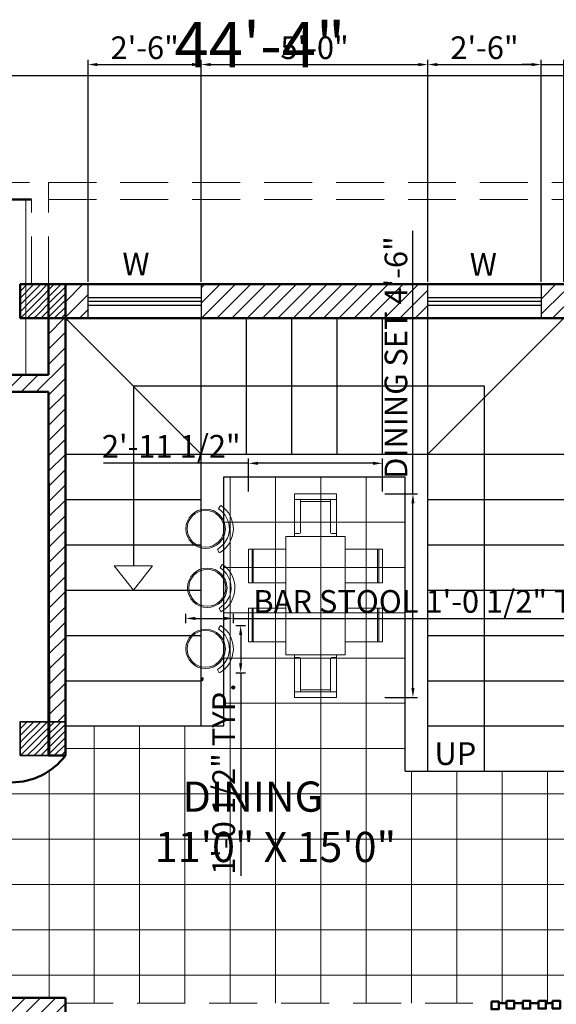
# Model space of a CAD drawing. Units: millimetres. Extents: x 225995 to 227247, y 225507 to 226008.
# Tile 3 of 23: x 226236 to 226378, y 225743 to 226004. Entities that reach past the tile are written whole.
import ezdxf

# ---------------------------------------------------------------- set-up
doc = ezdxf.new("R2010")
doc.units = ezdxf.units.MM
doc.linetypes.add('DASHED', pattern=[19.05, 12.7, -6.35])
for name, color, linetype, lineweight in [('A-ANNO-DIMS', 2, 'Continuous', 18), ('A-ANNO-TEXT', 3, 'Continuous', 18), ('A-AREA-IDEN', 30, 'Continuous', 18), ('A-COLS', 40, 'Continuous', 35), ('A-FLOR-PATT', 8, 'Continuous', 13), ('A-FLOR-STRS', 141, 'Continuous', 25), ('A-FURN', 9, 'Continuous', 18), ('A-GLAZ', 4, 'Continuous', 25), ('A-WALL', 7, 'Continuous', 50), ('A-WALL-OVHD', 1, 'DASHED', 18), ('A-WALL-PATT', 8, 'Continuous', 13)]:
    doc.layers.add(name, color=color, linetype=linetype, lineweight=lineweight)
doc.styles.get("Standard").update_dxf_attribs({"font": 'arial.ttf'})
doc.dimstyles.new('ISO-25', dxfattribs={"dimtxt": 6, "dimasz": 2.5, "dimexe": 1.25, "dimexo": 0.625, "dimtad": 1, "dimdec": 0, "dimlunit": 3, "dimtxsty": 'Standard', "dimcen": 2.5, "dimadec": 0, "dimazin": 0, "dimtfac": 1, "dimtdec": 0, "dimtmove": 0, "dimatfit": 3, "dimfxl": 1, "dimarcsym": 0})
pattern_1 = [(45, (-144, 118.1361), (-0.898025612, 0.898025612), [])]
pattern_2 = [(45, (-144, 234), (-0.898025612, 0.898025612), [])]

# ---------------------------------------------------------------- blocks, each defined once
blk = doc.blocks.new('A$C2A521B94')
for p, q in [((-548, 0, -343), (-548, 441, -343)), ((-548, 441, -343), (-150, 441, -343)), ((-548, 398, -343), (-150, 398, -343)), ((-548, 385, -343), (-150, 385, -343)), ((-150, 441, -343), (-150, 0, -343)), ((548, 441, -343), (150, 441, -343)), ((150, 441, -343), (150, 0, -343)), ((548, 398, -343), (150, 398, -343)), ((548, 385, -343), (150, 385, -343)), ((548, 0, -343), (548, 441, -343)), ((700, 0), (-700, 0)), ((-700, 0), (-700, -700)), ((700, -700), (700, 0)), ((-700, -103), (-1204, -103)), ((-1204, -103), (-1204, -597)), ((-1137, -103), (-1137, -597)), ((-733, -103), (-733, -157)), ((700, -103), (1204, -103)), ((733, -103), (733, -157)), ((1137, -103), (1137, -597)), ((1204, -103), (1204, -597)), ((-748, -172), (-1137, -172)), ((-1113, -172), (-1113, -528)), ((748, -172), (1137, -172)), ((1113, -172), (1113, -528)), ((-748, -528), (-1137, -528)), ((-733, -597), (-733, -543)), ((733, -597), (733, -543)), ((748, -528), (1137, -528)), ((-1204, -597), (-700, -597)), ((1204, -597), (700, -597)), ((-700, -700), (700, -700)), ((-548, -700, -343), (-548, -1141, -343)), ((-150, -1141, -343), (-150, -700, -343)), ((150, -1141, -343), (150, -700, -343)), ((548, -700, -343), (548, -1141, -343)), ((-548, -1085, -343), (-150, -1085, -343)), ((-548, -1098, -343), (-150, -1098, -343)), ((-548, -1141, -343), (-150, -1141, -343)), ((548, -1085, -343), (150, -1085, -343)), ((548, -1098, -343), (150, -1098, -343)), ((548, -1141, -343), (150, -1141, -343))]:
    blk.add_line(p, q)
for centre, start, end in [((-748, -157), 270, 0), ((748, -157), 180, 270), ((-748, -543), 0, 90), ((748, -543), 90, 180)]:
    blk.add_arc(centre, 14.7, start, end)
blk = doc.blocks.new('A$C2872593E')
for p, q in [((35, 351), (0, 373)), ((471, 339), (508, 360))]:
    blk.add_line(p, q)
for radius in [212, 198]:
    blk.add_circle((250, 213), radius)
for centre, radius, start, end in [((250, 213), 298, 29.6321, 146.9853), ((250, 213), 255, 29.6321, 147.1495), ((1, 374), 0.85, 146.9853, 237.1495), ((1, 374), 0.85, 146.9853, 237.1495)]:
    blk.add_arc(centre, radius, start, end)
at = {"flags": 9}
for tag in ['ZSIZE', 'YSIZE', 'XSIZE']:
    blk.add_attdef(tag, (257, 228), '', height=0.5, rotation=178.4267, dxfattribs=at)
blk = doc.blocks.new('A$C005B7AE8')
for p, q in [((0, 0.7), (0, 0.57)), ((0.03, 0.71), (0.03, 0.58)), ((0.46, 0.74), (0.04, 0.74)), ((0.44, 0.74), (0.06, 0.74)), ((0.38, 0.48), (0.12, 0.48)), ((0.13, 0.5), (0.15, 0.5)), ((0.14, 0.49), (0.14, 0.52)), ((0.14, 0.48), (0.14, 0.5)), ((0.15, 0.5), (0.15, 0.48)), ((0.35, 0.5), (0.35, 0.48)), ((0.37, 0.5), (0.35, 0.5)), ((0.36, 0.49), (0.36, 0.52)), ((0.36, 0.48), (0.36, 0.5)), ((0.47, 0.71), (0.47, 0.58)), ((0.5, 0.7), (0.5, 0.57))]:
    blk.add_line(p, q)
for centre in [(0.14, 0.55), (0.36, 0.55)]:
    blk.add_circle(centre, 0.00582)
for centre, radius, start, end in [((0.04, 0.7), 0.04, 90, 180), ((0.92, 0.57), 0.916, 179.9528, 200.6123), ((0.15, 0.45), 0.158, 140.1815, 162.8478), ((0.06, 0.71), 0.03, 90, 180), ((0.04, 0.58), 0.01, 180, 265.0115), ((0.25, 2.99), 2.42, 265.0115, 274.9885), ((0.14, 0.5), 0.00615, 5.1568, 174.8432), ((0.36, 0.5), 0.00615, 5.1568, 174.8432), ((0.44, 0.71), 0.03, 0, 90), ((-0.42, 0.57), 0.916, 339.3877, 0.0472), ((0.46, 0.7), 0.04, 0, 90), ((0.46, 0.58), 0.01, 274.9885, 0), ((0.35, 0.45), 0.158, 17.1522, 39.8185)]:
    blk.add_arc(centre, radius, start, end)
blk.add_ellipse((0.25, 0.28), major_axis=(0, -0.281), ratio=0.685919, start_param=3.915332, end_param=8.651039)
for centre, major_axis, ratio in [((0.25, 0.26), (0, -0.214), 0.687861), ((0.25, 0.25), (0, -0.0607), 0.657164)]:
    blk.add_ellipse(centre, major_axis=major_axis, ratio=ratio)
blk.add_open_spline([(0.13, 0.48), (0.12, 0.47), (0.12, 0.46), (0.11, 0.44), (0.1, 0.43), (0.09, 0.41), (0.09, 0.39), (0.08, 0.37), (0.08, 0.35), (0.07, 0.32), (0.07, 0.31), (0.07, 0.28), (0.07, 0.27), (0.07, 0.24), (0.08, 0.22), (0.08, 0.19), (0.09, 0.18), (0.09, 0.15), (0.1, 0.14), (0.11, 0.12), (0.12, 0.11), (0.13, 0.09), (0.14, 0.08), (0.15, 0.06), (0.16, 0.05), (0.18, 0.04), (0.19, 0.03), (0.2, 0.02), (0.21, 0.02), (0.23, 0.02), (0.24, 0.01), (0.26, 0.01), (0.27, 0.02), (0.29, 0.02), (0.3, 0.02), (0.31, 0.03), (0.32, 0.04), (0.34, 0.05), (0.35, 0.06), (0.36, 0.08), (0.37, 0.09), (0.38, 0.11), (0.39, 0.12), (0.4, 0.14), (0.41, 0.15), (0.41, 0.18), (0.42, 0.19), (0.42, 0.22), (0.43, 0.24), (0.43, 0.27), (0.43, 0.28), (0.43, 0.31), (0.43, 0.32), (0.42, 0.35), (0.42, 0.37), (0.41, 0.39), (0.41, 0.41), (0.4, 0.43), (0.39, 0.44), (0.38, 0.46), (0.38, 0.47), (0.37, 0.48)], degree=3, knots=[3.915332, 3.915332, 3.915332, 3.915332, 4.014441, 4.014441, 4.176505, 4.176505, 4.338569, 4.338569, 4.500633, 4.500633, 4.662697, 4.662697, 4.824761, 4.824761, 4.986825, 4.986825, 5.148889, 5.148889, 5.310953, 5.310953, 5.473017, 5.473017, 5.635081, 5.635081, 5.797146, 5.797146, 5.95921, 5.95921, 6.121274, 6.121274, 6.283338, 6.283338, 6.445402, 6.445402, 6.607466, 6.607466, 6.76953, 6.76953, 6.931594, 6.931594, 7.093658, 7.093658, 7.255722, 7.255722, 7.417786, 7.417786, 7.57985, 7.57985, 7.741915, 7.741915, 7.903979, 7.903979, 8.066043, 8.066043, 8.228107, 8.228107, 8.390171, 8.390171, 8.552235, 8.552235, 8.651039, 8.651039, 8.651039, 8.651039])
blk = doc.blocks.new('*D68')
at = {"layer": 'A-ANNO-DIMS', "color": 0, "lineweight": -2, "transparency": 16777216}
for p, q in [((226033.88, 225961.4), (226033.88, 225990.31)), ((226039.88, 225989.06), (226559.88, 225989.06)), ((226565.88, 225961.4), (226565.88, 225990.31))]:
    blk.add_line(p, q, dxfattribs=at)
at = {"layer": 'A-ANNO-DIMS', "color": 0, "transparency": 16777216}
for points in [[(226039.88, 225990.06), (226039.88, 225988.06), (226033.88, 225989.06)], [(226559.88, 225990.06), (226559.88, 225988.06), (226565.88, 225989.06)]]:
    blk.add_solid(points, dxfattribs=at)
at = {"layer": 'Defpoints', "color": 0, "transparency": 16777216}
for p in [(226565.88, 225989.06), (226033.88, 225960.77), (226565.88, 225960.77)]:
    blk.add_point(p, dxfattribs=at)
at = {"layer": 'A-ANNO-DIMS', "color": 0, "transparency": 16777216, "insert": (226299.88, 225995.68), "char_height": 12, "attachment_point": 5}
blk.add_mtext('44\'-4"', dxfattribs=at)
blk = doc.blocks.new('*D81')
at = {"layer": 'A-ANNO-DIMS', "color": 0, "lineweight": -2, "transparency": 16777216}
for p, q in [((226280.28, 225843.99), (226280.28, 225846.51)), ((226282.78, 225845.26), (226290.41, 225845.26)), ((226292.91, 225843.99), (226292.91, 225846.51)), ((226292.91, 225845.26), (226397.25, 225845.26))]:
    blk.add_line(p, q, dxfattribs=at)
at = {"layer": 'A-ANNO-DIMS', "color": 0, "transparency": 16777216}
for points in [[(226282.78, 225845.68), (226282.78, 225844.84), (226280.28, 225845.26)], [(226290.41, 225845.68), (226290.41, 225844.84), (226292.91, 225845.26)]]:
    blk.add_solid(points, dxfattribs=at)
at = {"layer": 'Defpoints', "color": 0, "transparency": 16777216}
for p in [(226292.91, 225845.26), (226280.28, 225843.36), (226292.91, 225843.36)]:
    blk.add_point(p, dxfattribs=at)
at = {"layer": 'A-ANNO-DIMS', "color": 0, "transparency": 16777216, "insert": (226346.33, 225848.99), "char_height": 6, "attachment_point": 5}
blk.add_mtext('BAR STOOL 1\'-0 1/2" TYP.', dxfattribs=at)
blk = doc.blocks.new('*D82')
at = {"layer": 'A-ANNO-DIMS', "color": 0, "lineweight": -2, "transparency": 16777216}
for p, q in [((226293.54, 225843.36), (226296.06, 225843.36)), ((226294.81, 225840.86), (226294.81, 225833.34)), ((226293.54, 225830.84), (226296.06, 225830.84)), ((226294.81, 225830.84), (226294.81, 225777.1))]:
    blk.add_line(p, q, dxfattribs=at)
at = {"layer": 'A-ANNO-DIMS', "color": 0, "transparency": 16777216}
for points in [[(226294.39, 225840.86), (226295.22, 225840.86), (226294.81, 225843.36)], [(226294.39, 225833.34), (226295.22, 225833.34), (226294.81, 225830.84)]]:
    blk.add_solid(points, dxfattribs=at)
at = {"layer": 'Defpoints', "color": 0, "transparency": 16777216}
for p in [(226292.91, 225843.36), (226292.91, 225830.84), (226294.81, 225830.84)]:
    blk.add_point(p, dxfattribs=at)
at = {"layer": 'A-ANNO-DIMS', "color": 0, "transparency": 16777216, "insert": (226291.08, 225802.72), "char_height": 6, "attachment_point": 5, "rotation": 90}
blk.add_mtext('1\'-0 1/2" TYP.', dxfattribs=at)
blk = doc.blocks.new('*D87')
at = {"layer": 'A-ANNO-DIMS', "color": 0, "lineweight": -2, "transparency": 16777216}
for p, q in [((226340.43, 225878.26), (226340.43, 225947.96)), ((226332.97, 225878.26), (226341.68, 225878.26)), ((226340.43, 225826.84), (226340.43, 225875.76)), ((226332.97, 225824.34), (226341.68, 225824.34))]:
    blk.add_line(p, q, dxfattribs=at)
at = {"layer": 'A-ANNO-DIMS', "color": 0, "transparency": 16777216}
for points in [[(226340.02, 225875.76), (226340.85, 225875.76), (226340.43, 225878.26)], [(226340.02, 225826.84), (226340.85, 225826.84), (226340.43, 225824.34)]]:
    blk.add_solid(points, dxfattribs=at)
at = {"layer": 'Defpoints', "color": 0, "transparency": 16777216}
for p in [(226332.34, 225878.26), (226340.43, 225878.26), (226332.34, 225824.34)]:
    blk.add_point(p, dxfattribs=at)
at = {"layer": 'A-ANNO-DIMS', "color": 0, "transparency": 16777216, "insert": (226336.71, 225914.36), "char_height": 6, "attachment_point": 5, "rotation": 90}
blk.add_mtext('DINING SET 4\'-6"', dxfattribs=at)
blk = doc.blocks.new('*D88')
at = {"layer": 'A-ANNO-DIMS', "color": 0, "lineweight": -2, "transparency": 16777216}
for p, q in [((226296.89, 225878.89), (226296.89, 225887.6)), ((226332.34, 225878.89), (226332.34, 225887.6)), ((226296.89, 225886.35), (226258.44, 225886.35)), ((226329.84, 225886.35), (226299.39, 225886.35))]:
    blk.add_line(p, q, dxfattribs=at)
at = {"layer": 'A-ANNO-DIMS', "color": 0, "transparency": 16777216}
for points in [[(226299.39, 225886.77), (226299.39, 225885.93), (226296.89, 225886.35)], [(226329.84, 225886.77), (226329.84, 225885.93), (226332.34, 225886.35)]]:
    blk.add_solid(points, dxfattribs=at)
at = {"layer": 'Defpoints', "color": 0, "transparency": 16777216}
for p in [(226296.89, 225886.35), (226296.89, 225878.26), (226332.34, 225878.26)]:
    blk.add_point(p, dxfattribs=at)
at = {"layer": 'A-ANNO-DIMS', "color": 0, "transparency": 16777216, "insert": (226276.42, 225890.08), "char_height": 6, "attachment_point": 5}
blk.add_mtext('2\'-11 1/2"', dxfattribs=at)
blk = doc.blocks.new('*D93')
at = {"layer": 'A-ANNO-DIMS', "color": 0, "lineweight": -2, "transparency": 16777216}
for p, q in [((226254.38, 225934.4), (226254.38, 225993.22)), ((226256.88, 225991.97), (226281.88, 225991.97)), ((226284.38, 225934.4), (226284.38, 225993.22))]:
    blk.add_line(p, q, dxfattribs=at)
at = {"layer": 'A-ANNO-DIMS', "color": 0, "transparency": 16777216}
for points in [[(226256.88, 225992.39), (226256.88, 225991.56), (226254.38, 225991.97)], [(226281.88, 225992.39), (226281.88, 225991.56), (226284.38, 225991.97)]]:
    blk.add_solid(points, dxfattribs=at)
at = {"layer": 'Defpoints', "color": 0, "transparency": 16777216}
for p in [(226284.38, 225991.97), (226254.38, 225933.77), (226284.38, 225933.77)]:
    blk.add_point(p, dxfattribs=at)
at = {"layer": 'A-ANNO-DIMS', "color": 0, "transparency": 16777216, "insert": (226269.38, 225995.66), "char_height": 6, "attachment_point": 5}
blk.add_mtext('2\'-6"', dxfattribs=at)
blk = doc.blocks.new('*D94')
at = {"layer": 'A-ANNO-DIMS', "color": 0, "lineweight": -2, "transparency": 16777216}
for p, q in [((226284.38, 225934.4), (226284.38, 225993.22)), ((226286.88, 225991.97), (226341.88, 225991.97)), ((226344.38, 225934.4), (226344.38, 225993.22))]:
    blk.add_line(p, q, dxfattribs=at)
at = {"layer": 'A-ANNO-DIMS', "color": 0, "transparency": 16777216}
for points in [[(226286.88, 225992.39), (226286.88, 225991.56), (226284.38, 225991.97)], [(226341.88, 225992.39), (226341.88, 225991.56), (226344.38, 225991.97)]]:
    blk.add_solid(points, dxfattribs=at)
at = {"layer": 'Defpoints', "color": 0, "transparency": 16777216}
for p in [(226344.38, 225991.97), (226284.38, 225933.77), (226344.38, 225933.77)]:
    blk.add_point(p, dxfattribs=at)
at = {"layer": 'A-ANNO-DIMS', "color": 0, "transparency": 16777216, "insert": (226314.38, 225995.66), "char_height": 6, "attachment_point": 5}
blk.add_mtext('5\'-0"', dxfattribs=at)
blk = doc.blocks.new('*D95')
at = {"layer": 'A-ANNO-DIMS', "color": 0, "lineweight": -2, "transparency": 16777216}
for p, q in [((226344.38, 225934.4), (226344.38, 225993.22)), ((226346.88, 225991.97), (226371.88, 225991.97)), ((226374.38, 225934.4), (226374.38, 225993.22))]:
    blk.add_line(p, q, dxfattribs=at)
at = {"layer": 'A-ANNO-DIMS', "color": 0, "transparency": 16777216}
for points in [[(226346.88, 225992.39), (226346.88, 225991.56), (226344.38, 225991.97)], [(226371.88, 225992.39), (226371.88, 225991.56), (226374.38, 225991.97)]]:
    blk.add_solid(points, dxfattribs=at)
at = {"layer": 'Defpoints', "color": 0, "transparency": 16777216}
for p in [(226374.38, 225991.97), (226344.38, 225933.77), (226374.38, 225933.77)]:
    blk.add_point(p, dxfattribs=at)
at = {"layer": 'A-ANNO-DIMS', "color": 0, "transparency": 16777216, "insert": (226359.38, 225995.66), "char_height": 6, "attachment_point": 5}
blk.add_mtext('2\'-6"', dxfattribs=at)
blk = doc.blocks.new('*D96')
at = {"layer": 'A-ANNO-DIMS', "color": 0, "lineweight": -2, "transparency": 16777216}
for p, q in [((226371.88, 225991.97), (226369.38, 225991.97)), ((226374.38, 225934.4), (226374.38, 225993.22)), ((226374.38, 225991.97), (226380.38, 225991.97)), ((226380.38, 225934.4), (226380.38, 225993.22)), ((226382.88, 225991.97), (226402.58, 225991.97))]:
    blk.add_line(p, q, dxfattribs=at)
at = {"layer": 'A-ANNO-DIMS', "color": 0, "transparency": 16777216}
for points in [[(226371.88, 225992.39), (226371.88, 225991.56), (226374.38, 225991.97)], [(226382.88, 225992.39), (226382.88, 225991.56), (226380.38, 225991.97)]]:
    blk.add_solid(points, dxfattribs=at)
at = {"layer": 'Defpoints', "color": 0, "transparency": 16777216}
for p in [(226380.38, 225991.97), (226374.38, 225933.77), (226380.38, 225933.77)]:
    blk.add_point(p, dxfattribs=at)
at = {"layer": 'A-ANNO-DIMS', "color": 0, "transparency": 16777216, "insert": (226393.98, 225995.66), "char_height": 6, "attachment_point": 5}
blk.add_mtext('0\'-6"', dxfattribs=at)

msp = doc.modelspace()

# ---------------------------------------------------------------- hatches: boundary and pattern name
at = {"layer": 'A-WALL-PATT'}
h = msp.add_hatch(dxfattribs=at)
h.set_pattern_fill('ANSI31', color=256, scale=0.4)
h.set_pattern_definition(pattern_2)
h.paths.add_polyline_path([(226240.88, 225933.77), (226236.38, 225933.77), (226236.38, 225929.27), (226240.88, 225929.27)])
h = msp.add_hatch(dxfattribs=at)
h.set_pattern_fill('ANSI31', color=256, scale=0.4)
h.set_pattern_definition(pattern_2)
h.paths.add_polyline_path([(226248.38, 225933.77), (226240.88, 225933.77), (226240.88, 225929.27), (226248.38, 225929.27)])
h = msp.add_hatch(dxfattribs=at)
h.set_pattern_fill('ANSI31', color=256, scale=0.9)
h.paths.add_polyline_path([(226254.38, 225933.77), (226248.38, 225933.77), (226248.38, 225924.77), (226254.38, 225924.77)])
h = msp.add_hatch(dxfattribs=at)
h.set_pattern_fill('ANSI31', color=256, scale=0.9)
h.paths.add_polyline_path([(226344.38, 225933.77), (226284.38, 225933.77), (226284.38, 225924.77), (226344.38, 225924.77)])
h = msp.add_hatch(dxfattribs=at)
h.set_pattern_fill('ANSI31', color=256, scale=0.9)
h.paths.add_polyline_path([(226380.38, 225933.77), (226374.38, 225933.77), (226374.38, 225924.77), (226380.38, 225924.77)])
h = msp.add_hatch(dxfattribs=at)
h.set_pattern_fill('ANSI31', color=256, scale=0.4)
h.set_pattern_definition(pattern_2)
h.paths.add_polyline_path([(226240.88, 225929.27), (226236.38, 225929.27), (226236.38, 225924.77), (226240.88, 225924.77)])
h = msp.add_hatch(dxfattribs=at)
h.set_pattern_fill('ANSI31', color=256, scale=0.4)
h.set_pattern_definition(pattern_2)
h.paths.add_polyline_path([(226248.38, 225929.27), (226240.88, 225929.27), (226240.88, 225924.77), (226248.38, 225924.77)])
h = msp.add_hatch(dxfattribs=at)
h.set_pattern_fill('ANSI31', color=256, scale=0.9)
h.paths.add_polyline_path([(226248.38, 225924.77), (226243.88, 225924.77), (226243.88, 225909.77), (226219.88, 225909.77), (226219.88, 225905.27), (226243.88, 225905.27), (226244.03, 225817.91), (226248.38, 225817.91)])
h = msp.add_hatch(dxfattribs=at)
h.set_pattern_fill('ANSI31', color=256, scale=0.4)
h.set_pattern_definition(pattern_1)
h.paths.add_polyline_path([(226240.88, 225817.91), (226236.38, 225817.91), (226236.38, 225813.41), (226240.88, 225813.41)])
h = msp.add_hatch(dxfattribs=at)
h.set_pattern_fill('ANSI31', color=256, scale=0.4)
h.set_pattern_definition(pattern_1)
h.paths.add_polyline_path([(226248.38, 225817.91), (226240.88, 225817.91), (226240.88, 225813.41), (226248.38, 225813.41)])
h = msp.add_hatch(dxfattribs=at)
h.set_pattern_fill('ANSI31', color=256, scale=0.4)
h.set_pattern_definition(pattern_1)
h.paths.add_polyline_path([(226240.88, 225813.41), (226236.38, 225813.41), (226236.38, 225808.91), (226240.88, 225808.91)])
h = msp.add_hatch(dxfattribs=at)
h.set_pattern_fill('ANSI31', color=256, scale=0.4)
h.set_pattern_definition(pattern_1)
h.paths.add_polyline_path([(226248.38, 225813.41), (226240.88, 225813.41), (226240.88, 225808.91), (226248.38, 225808.91)])
h = msp.add_hatch(dxfattribs=at)
h.set_pattern_fill('ANSI31', color=256, scale=0.9)
h.paths.add_polyline_path([(226111.88, 225740.27), (226248.38, 225740.27), (226248.38, 225744.77), (226188.38, 225744.77), (226188.38, 225756.77), (226183.88, 225756.77), (226183.88, 225744.77), (226111.88, 225744.77), (226111.88, 225762.77), (226102.88, 225762.77), (226102.88, 225702.77), (226111.88, 225702.77)])

# ---------------------------------------------------------------- linework, layer by layer
at = {"layer": 'A-COLS'}
for points in [[(226236.38, 225924.77), (226236.38, 225933.77), (226248.38, 225933.77), (226248.38, 225924.77)], [(226236.38, 225808.91), (226236.38, 225817.91), (226248.38, 225817.91), (226248.38, 225808.91)]]:
    msp.add_lwpolyline(points, close=True, dxfattribs=at)
at = {"layer": 'A-FLOR-PATT'}
for p, q in [((226292.05, 225882.77), (226292.05, 225743.31)), ((226304.05, 225882.77), (226304.05, 225743.31)), ((226316.05, 225882.77), (226316.05, 225743.31)), ((226328.05, 225882.77), (226328.05, 225743.31)), ((226290.38, 225870.77), (226338.38, 225870.77)), ((226290.38, 225858.77), (226338.38, 225858.77)), ((226290.38, 225846.77), (226338.38, 225846.77)), ((226290.38, 225834.77), (226338.38, 225834.77)), ((226290.38, 225822.77), (226338.38, 225822.77)), ((226256.05, 225816.77), (226256.05, 225743.31)), ((226268.05, 225816.77), (226268.05, 225743.31)), ((226280.05, 225816.77), (226280.05, 225743.31)), ((226248.38, 225810.77), (226338.38, 225810.77)), ((226244.05, 225804.83), (226244.05, 225744.77)), ((226340.05, 225804.77), (226340.05, 225743.31)), ((226352.05, 225804.77), (226352.05, 225743.31)), ((226364.05, 225804.77), (226364.05, 225743.31)), ((226376.05, 225804.77), (226376.05, 225743.31)), ((226219.88, 225798.77), (226380.38, 225798.77)), ((226219.88, 225786.77), (226380.38, 225786.77)), ((226219.88, 225774.77), (226380.38, 225774.77)), ((226219.88, 225762.77), (226380.38, 225762.77)), ((226219.88, 225750.77), (226380.38, 225750.77))]:
    msp.add_line(p, q, dxfattribs=at)
at = {"layer": 'A-FLOR-STRS'}
for p, q in [((226248.38, 225924.77), (226284.38, 225888.77)), ((226284.38, 225816.77), (226284.38, 225924.77)), ((226296.38, 225888.77), (226296.38, 225924.77)), ((226308.38, 225888.77), (226308.38, 225924.77)), ((226320.38, 225888.77), (226320.38, 225924.77)), ((226332.38, 225888.77), (226332.38, 225924.77)), ((226344.38, 225804.77), (226344.38, 225924.77)), ((226344.38, 225888.77), (226380.38, 225924.77)), ((226359.38, 225906.77), (226266.38, 225906.77)), ((226266.38, 225906.77), (226266.38, 225859.15)), ((226359.38, 225804.77), (226359.38, 225906.77)), ((226248.38, 225888.77), (226380.38, 225888.77)), ((226290.38, 225816.77), (226290.38, 225882.77)), ((226290.38, 225882.77), (226338.38, 225882.77)), ((226338.38, 225804.77), (226338.38, 225882.77)), ((226248.38, 225876.77), (226284.38, 225876.77)), ((226344.38, 225876.77), (226380.38, 225876.77)), ((226248.38, 225864.77), (226284.38, 225864.77)), ((226344.38, 225864.77), (226380.38, 225864.77)), ((226248.38, 225852.77), (226284.38, 225852.77)), ((226344.38, 225852.77), (226380.38, 225852.77)), ((226248.38, 225840.77), (226284.38, 225840.77)), ((226344.38, 225840.77), (226380.38, 225840.77)), ((226248.38, 225828.77), (226284.38, 225828.77)), ((226344.38, 225828.77), (226380.38, 225828.77)), ((226248.38, 225816.77), (226290.38, 225816.77)), ((226344.38, 225816.77), (226380.38, 225816.77)), ((226338.38, 225804.77), (226380.38, 225804.77))]:
    msp.add_line(p, q, dxfattribs=at)
at = {"layer": 'A-FURN'}
for p, q in [((226237.88, 225909.77), (226237.88, 225956.27)), ((226254.38, 225933.77), (226254.38, 225924.77)), ((226284.38, 225933.77), (226284.38, 225924.77)), ((226344.38, 225933.77), (226344.38, 225924.77)), ((226374.38, 225933.77), (226374.38, 225924.77)), ((226266.38, 225852.77), (226261.29, 225859.15)), ((226261.29, 225859.15), (226271.46, 225859.15)), ((226266.38, 225852.77), (226271.46, 225859.15))]:
    msp.add_line(p, q, dxfattribs=at)
at = {"layer": 'A-GLAZ'}
for p, q in [((226254.38, 225930.27), (226284.38, 225930.27)), ((226254.38, 225929.27), (226284.38, 225929.27)), ((226344.38, 225930.27), (226374.38, 225930.27)), ((226344.43, 225929.27), (226374.38, 225929.27)), ((226254.38, 225928.27), (226284.38, 225928.27)), ((226344.38, 225928.27), (226374.38, 225928.27))]:
    msp.add_line(p, q, dxfattribs=at)
for points in [[(226254.38, 225933.77), (226284.38, 225933.77), (226284.38, 225924.77), (226254.38, 225924.77)], [(226344.38, 225933.77), (226374.38, 225933.77), (226374.38, 225924.77), (226344.38, 225924.77)]]:
    msp.add_lwpolyline(points, close=True, dxfattribs=at)
at = {"layer": 'A-WALL'}
for p, q in [((226111.88, 225956.27), (226239.38, 225956.27)), ((226565.88, 225933.77), (226236.38, 225933.77)), ((226236.38, 225933.77), (226236.38, 225924.77)), ((226243.88, 225933.77), (226565.88, 225933.77)), ((226243.88, 225909.77), (226243.88, 225933.77)), ((226243.88, 225909.77), (226243.88, 225933.77)), ((226248.38, 225933.77), (226248.38, 225924.77)), ((226236.38, 225924.77), (226557.38, 225924.77)), ((226248.38, 225924.77), (226380.38, 225924.77)), ((226248.38, 225808.91), (226248.38, 225924.77)), ((226248.38, 225924.77), (226248.38, 225808.91)), ((226219.88, 225909.77), (226243.88, 225909.77)), ((226219.88, 225909.77), (226243.88, 225909.77)), ((226219.88, 225905.27), (226243.88, 225905.27)), ((226243.88, 225905.27), (226219.88, 225905.27)), ((226244.05, 225808.92), (226243.88, 225905.27)), ((226243.88, 225808.92), (226243.88, 225905.27)), ((226243.88, 225808.92), (226248.38, 225808.91)), ((226248.38, 225808.91), (226243.88, 225808.92)), ((226244.05, 225808.92), (226244.05, 225808.91)), ((226188.38, 225744.77), (226248.38, 225744.77)), ((226248.38, 225744.77), (226188.38, 225744.77)), ((226248.38, 225740.27), (226248.38, 225744.77)), ((226248.38, 225740.27), (226248.38, 225744.77)), ((226363.18, 225743.31), (226365.24, 225743.31)), ((226367.21, 225743.31), (226369.52, 225743.31)), ((226371.49, 225743.31), (226373.67, 225743.31)), ((226375.64, 225743.31), (226377.42, 225743.31))]:
    msp.add_line(p, q, dxfattribs=at)
for points in [[(226361.21, 225743.83), (226363.18, 225743.83), (226363.18, 225741.75), (226361.21, 225741.75)], [(226365.24, 225743.99), (226367.21, 225743.99), (226367.21, 225741.91), (226365.24, 225741.91)], [(226369.52, 225743.99), (226371.49, 225743.99), (226371.49, 225741.91), (226369.52, 225741.91)], [(226373.67, 225743.99), (226375.64, 225743.99), (226375.64, 225741.91), (226373.67, 225741.91)], [(226377.42, 225743.99), (226379.39, 225743.99), (226379.39, 225741.91), (226377.42, 225741.91)]]:
    msp.add_lwpolyline(points, close=True, dxfattribs=at)
msp.add_arc((226234.13, 225819.69), 17.87, 217.0967, 322.9033, dxfattribs=at)
at = {"layer": 'A-WALL-OVHD'}
for p, q in [((226111.88, 225960.77), (226243.88, 225960.77)), ((226243.88, 225960.77), (226565.88, 225960.77)), ((226243.88, 225933.77), (226243.88, 225960.77)), ((226111.88, 225956.27), (226239.38, 225956.27)), ((226239.38, 225933.77), (226239.38, 225956.27)), ((226243.88, 225956.27), (226561.38, 225956.27)), ((226248.38, 225743.31), (226361.21, 225743.31))]:
    msp.add_line(p, q, dxfattribs=at)

# ---------------------------------------------------------------- block references
at = {"layer": 'A-FURN'}
for name, p, xscale, yscale, zscale, rotation in [('A$C2A521B94', (226306.78, 225851.3), 0.0224019348229555, 0.0224019348229555, 0.0224019348229555, 90), ('A$C2872593E', (226280.28, 225875.18), 0.0246363059206613, 0.0246363059206613, 0.0246363059206613, 270), ('A$C2872593E', (226280.72, 225859.55), 0.0246363059206613, 0.0246363059206613, 0.0246363059206613, 270), ('A$C2872593E', (226280.28, 225843.36), 0.0246363059206613, 0.0246363059206613, 0.0246363059206613, 270)]:
    msp.add_blockref(name, p, dxfattribs=dict(at, xscale=xscale, yscale=yscale, zscale=zscale, rotation=rotation))
msp.add_blockref('A$C005B7AE8', (226284.38, 225828.77), dxfattribs=at)

# ---------------------------------------------------------------- texts
at = {"layer": 'A-ANNO-TEXT', "char_height": 6, "attachment_point": 1}
for s, insert in [('   W', (226257.98, 225942.16)), ('   W', (226349.97, 225942.03)), ('   UP', (226340.63, 225812.45))]:
    msp.add_mtext_dynamic_manual_height_columns(s, width=24.8115, gutter_width=12.5, heights=[0], dxfattribs=dict(at, insert=insert))
at = {"layer": 'A-AREA-IDEN', "insert": (226267.19, 225802.06), "char_height": 8, "attachment_point": 1}
msp.add_mtext_dynamic_manual_height_columns('     DINING\\P  11\'0" X 15\'0"', width=85.4795, gutter_width=12.5, heights=[0], dxfattribs=at)

# ---------------------------------------------------------------- dimensions: what is measured, and where the dimension line sits
at = {"layer": 'A-ANNO-DIMS'}
for base, p1, p2, override, picture, middle in [((226565.88, 225989.06), (226033.88, 225960.77), (226565.88, 225960.77), {"dimtxt": 12, "dimasz": 6, "dimclrd": 0, "dimclre": 0, "dimclrt": 0}, '*D68', (226299.88, 225995.68)), ((226284.38, 225991.97), (226254.38, 225933.77), (226284.38, 225933.77), {"dimdec": 1, "dimlfac": 1, "dimrnd": 0, "dimzin": 1, "dimdsep": 46, "dimlunit": 4, "dimfrac": 2}, '*D93', (226269.38, 225995.66)), ((226344.38, 225991.97), (226284.38, 225933.77), (226344.38, 225933.77), {"dimdec": 1, "dimlfac": 1, "dimrnd": 0, "dimzin": 1, "dimdsep": 46, "dimlunit": 4, "dimfrac": 2}, '*D94', (226314.38, 225995.66)), ((226374.38, 225991.97), (226344.38, 225933.77), (226374.38, 225933.77), {"dimdec": 1, "dimlfac": 1, "dimrnd": 0, "dimzin": 1, "dimdsep": 46, "dimlunit": 4, "dimfrac": 2}, '*D95', (226359.38, 225995.66)), ((226380.38, 225991.97), (226374.38, 225933.77), (226380.38, 225933.77), {"dimdec": 1, "dimlfac": 1, "dimrnd": 0, "dimzin": 1, "dimdsep": 46, "dimlunit": 4, "dimfrac": 2}, '*D96', (226393.98, 225995.66))]:
    dim = msp.add_linear_dim(base=base, p1=p1, p2=p2, dimstyle='ISO-25', override=override, dxfattribs=at)
    dim.commit()
    dim.dimension.update_dxf_attribs({"geometry": picture, "text_midpoint": middle})
for base, p1, p2, angle, text, picture, middle in [((226340.43, 225878.26), (226332.34, 225824.34), (226332.34, 225878.26), 90, 'DINING SET <>', '*D87', (226336.71, 225914.36)), ((226294.81, 225830.84), (226292.91, 225843.36), (226292.91, 225830.84), 270, '<> TYP.', '*D82', (226291.08, 225802.72))]:
    dim = msp.add_linear_dim(base=base, p1=p1, p2=p2, angle=angle, text=text, dimstyle='ISO-25', override={"dimdec": 1, "dimrnd": 0, "dimzin": 1, "dimlunit": 4, "dimfrac": 2}, dxfattribs=at)
    dim.commit()
    dim.dimension.update_dxf_attribs({"geometry": picture, "text_midpoint": middle})
dim = msp.add_linear_dim(base=(226296.8883, 225886.3515), p1=(226332.3439, 225878.2629), p2=(226296.8883, 225878.2629), angle=180, dimstyle='ISO-25', override={"dimdec": 1, "dimrnd": 0, "dimzin": 1, "dimlunit": 4, "dimfrac": 2}, dxfattribs=at)
dim.commit()
dim.dimension.update_dxf_attribs({"geometry": '*D88', "text_midpoint": (226276.416, 225890.0789)})
dim = msp.add_linear_dim(base=(226292.91, 225845.26), p1=(226280.28, 225843.36), p2=(226292.91, 225843.36), text='BAR STOOL <> TYP.', dimstyle='ISO-25', override={"dimdec": 1, "dimrnd": 0, "dimzin": 1, "dimlunit": 4, "dimfrac": 2}, dxfattribs=at)
dim.commit()
dim.dimension.update_dxf_attribs({"geometry": '*D81', "text_midpoint": (226346.33, 225848.99)})

doc.saveas('drawing.dxf')
